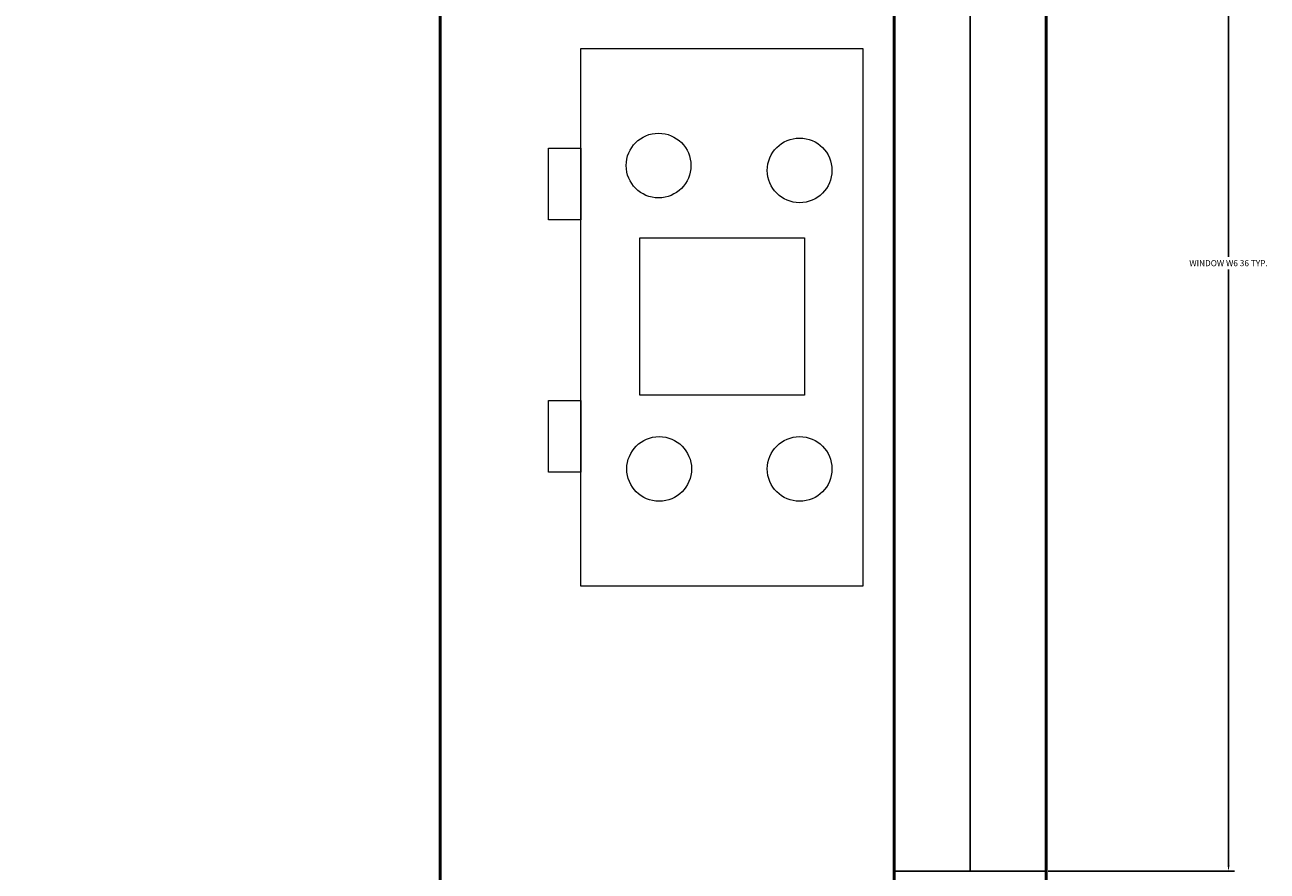
# Model space of a CAD drawing. Units: inches. Extents: x 1901 to 2863, y 888 to 2433.
# Tile 87 of 91: x 2723 to 2759, y 2027 to 2052. Entities that reach past the tile are written whole.
import ezdxf

# ---------------------------------------------------------------- set-up
doc = ezdxf.new("R2010")
doc.units = ezdxf.units.IN
for name, color, linetype, lineweight in [('A-ANNO-DIMS', 2, 'Continuous', 18), ('A-FLOR-FIXT', 9, 'Continuous', 18), ('A-GLAZ', 3, 'Continuous', 25), ('A-WALL', 7, 'Continuous', 50), ('A-WALL-PATT', 8, 'Continuous', 13)]:
    doc.layers.add(name, color=color, linetype=linetype, lineweight=lineweight)
doc.styles.get("Standard").update_dxf_attribs({"font": 'arial.ttf'})
doc.dimstyles.get("Standard").update_dxf_attribs({"dimtxt": 0.18, "dimasz": 0.18, "dimexe": 0.18, "dimexo": 0.0625, "dimgap": 0.09, "dimtad": 0, "dimtih": 1, "dimtoh": 1, "dimdec": 4, "dimzin": 0, "dimdsep": 46, "dimtxsty": 'Standard', "dimcen": 0.09, "dimadec": 0, "dimazin": 0, "dimtfac": 1, "dimtdec": 4, "dimtofl": 0, "dimtmove": 0, "dimatfit": 3, "dimfxl": 1, "dimtolj": 1, "dimtzin": 0, "dimarcsym": 0})

# ---------------------------------------------------------------- blocks, each defined once
blk = doc.blocks.new('WIN-36-5')
for p, q in [((0, 36), (4.5, 36)), ((4.5, 36), (2.25, 36)), ((2.25, 36), (2.25, 0)), ((2.25, 0), (0, 0)), ((0, 0), (4.5, 0))]:
    blk.add_line(p, q)
blk = doc.blocks.new('*D29')
at = {"layer": 'A-ANNO-DIMS', "color": 0, "lineweight": -2, "transparency": 16777216}
for p, q in [((2752.989, 2063.429), (2758.506, 2063.429)), ((2758.326, 2063.249), (2758.326, 2045.612)), ((2758.326, 2027.609), (2758.326, 2045.245)), ((2752.989, 2027.429), (2758.506, 2027.429))]:
    blk.add_line(p, q, dxfattribs=at)
at = {"layer": 'A-ANNO-DIMS', "color": 0, "transparency": 16777216}
for points in [[(2758.296, 2063.249), (2758.356, 2063.249), (2758.326, 2063.429)], [(2758.296, 2027.609), (2758.356, 2027.609), (2758.326, 2027.429)]]:
    blk.add_solid(points, dxfattribs=at)
at = {"layer": 'Defpoints', "color": 0, "transparency": 16777216}
for p in [(2752.926, 2063.429), (2758.326, 2063.429), (2752.926, 2027.429)]:
    blk.add_point(p, dxfattribs=at)
at = {"layer": 'A-ANNO-DIMS', "color": 0, "transparency": 16777216, "insert": (2758.326, 2045.429), "char_height": 0.18, "attachment_point": 5}
blk.add_mtext('\\A1;WINDOW W6 36 TYP.', dxfattribs=at)
blk = doc.blocks.new('*D30')
at = {"layer": 'A-ANNO-DIMS', "color": 0, "lineweight": -2, "transparency": 16777216}
for p, q in [((2748.426, 2027.366), (2748.426, 2021.849)), ((2752.926, 2027.366), (2752.926, 2021.849)), ((2748.606, 2022.029), (2750.218, 2022.029)), ((2752.746, 2022.029), (2751.134, 2022.029))]:
    blk.add_line(p, q, dxfattribs=at)
at = {"layer": 'A-ANNO-DIMS', "color": 0, "transparency": 16777216}
for points in [[(2748.606, 2022.059), (2748.606, 2021.999), (2748.426, 2022.029)], [(2752.746, 2022.059), (2752.746, 2021.999), (2752.926, 2022.029)]]:
    blk.add_solid(points, dxfattribs=at)
at = {"layer": 'Defpoints', "color": 0, "transparency": 16777216}
for p in [(2748.426, 2027.429), (2752.926, 2027.429), (2752.926, 2022.029)]:
    blk.add_point(p, dxfattribs=at)
at = {"layer": 'A-ANNO-DIMS', "color": 0, "transparency": 16777216, "insert": (2750.676, 2022.029), "char_height": 0.18, "attachment_point": 5}
blk.add_mtext('\\A1;5 TYP.', dxfattribs=at)

msp = doc.modelspace()

# ---------------------------------------------------------------- hatches: boundary and pattern name
at = {"layer": 'A-WALL-PATT'}
h = msp.add_hatch(dxfattribs=at)
h.set_pattern_fill('ANSI32', color=256)
h.paths.add_polyline_path([(2192.501, 2274.134), (2141.264, 2274.134), (2141.264, 2269.634), (2192.501, 2269.634)])
h.paths.add_polyline_path([(2259.926, 2274.134), (2216.501, 2274.134), (2216.501, 2269.634), (2255.426, 2269.634), (2255.426, 2214.634), (2250.809, 2214.634), (2250.809, 2210.134), (2259.926, 2210.134), (2259.926, 2215.134), (2271.756, 2215.134), (2271.756, 2217.384), (2271.756, 2219.634), (2259.926, 2219.634)])
h.paths.add_polyline_path([(2171.426, 2269.634), (2166.926, 2269.634), (2166.926, 2219.634), (2121.238, 2219.634), (2121.238, 2215.134), (2166.926, 2215.134), (2166.926, 2083.134), (2161.807, 2083.134), (2161.807, 2078.634), (2171.426, 2078.634), (2176.996, 2078.634), (2176.996, 2080.884), (2176.996, 2083.134), (2171.426, 2083.134), (2171.426, 2210.134), (2230.912, 2210.134), (2230.912, 2212.384), (2230.912, 2214.634), (2171.426, 2214.634)])
h.paths.add_polyline_path([(2117.264, 2274.134), (2089.426, 2274.134), (2089.426, 2219.634), (2081.136, 2219.634), (2081.136, 2215.134), (2089.426, 2215.134), (2098.004, 2215.134), (2098.004, 2217.384), (2098.004, 2219.634), (2093.926, 2219.634), (2093.926, 2269.634), (2117.264, 2269.634), (2117.264, 2271.884)])
h.paths.add_polyline_path([(2343.426, 2219.634), (2329.295, 2219.634), (2329.295, 2215.134), (2338.926, 2215.134), (2338.926, 2184.739), (2343.426, 2184.739)])
h.paths.add_polyline_path([(2338.926, 2083.134), (2329.295, 2083.134), (2208.966, 2083.134), (2208.966, 2078.634), (2338.926, 2078.634)])
h.paths.add_polyline_path([(2343.426, 2136.739), (2338.926, 2136.739), (2338.926, 1872.634), (2343.426, 1872.634)])
h.paths.add_polyline_path([(2343.426, 1863.634), (2397.68, 1863.634), (2397.68, 1821.634), (2384.138, 1821.634), (2384.138, 1812.634), (2418.33, 1812.634), (2418.33, 1817.134), (2418.33, 1821.634), (2406.68, 1821.634), (2406.68, 1863.634), (2459.499, 1863.634), (2459.499, 1821.634), (2447.138, 1821.634), (2447.138, 1812.634), (2459.499, 1812.634), (2468.499, 1812.634), (2468.499, 1872.634), (2394.426, 1872.634), (2334.426, 1872.634), (2334.426, 1812.634), (2343.426, 1812.634), (2353.251, 1812.634), (2353.251, 1821.634), (2343.426, 1821.634)])
h.paths.add_polyline_path([(2510.014, 1872.634), (2468.499, 1872.634), (2468.499, 1868.134), (2510.014, 1868.134)])
h.paths.add_polyline_path([(2514.009, 1817.134), (2468.499, 1817.134), (2468.499, 1812.634), (2482.114, 1812.634), (2482.114, 1800.606), (2486.614, 1800.606), (2486.614, 1812.634), (2514.009, 1812.634)])
h.paths.add_polyline_path([(2299.247, 1814.884), (2299.247, 1817.134), (2295.926, 1817.134), (2295.926, 1854.169), (2293.676, 1854.169), (2291.426, 1854.169), (2291.426, 1817.134), (2266.109, 1817.134), (2266.109, 1812.634), (2299.247, 1812.634)])
h.paths.add_polyline_path([(2218.109, 1817.134), (2206.46, 1817.134), (2171.426, 1817.134), (2171.426, 1949.134), (2190.1, 1949.134), (2190.1, 1953.634), (2163.468, 1953.634), (2163.468, 1949.134), (2166.926, 1949.134), (2166.926, 1817.134), (2114.297, 1817.134), (2114.297, 1812.634), (2218.109, 1812.634)])
h.paths.add_polyline_path([(2029.426, 1970.922), (2024.926, 1970.922), (2024.926, 1912.717), (2029.426, 1912.717)])
h.paths.add_polyline_path([(2132.297, 1953.634), (2113.926, 1953.634), (2113.926, 1975.888), (2111.676, 1975.888), (2109.426, 1975.888), (2109.426, 1953.634), (2029.426, 1953.634), (2029.426, 1949.134), (2132.297, 1949.134)])
h.paths.add_polyline_path([(2029.426, 1853.606), (2029.31, 1853.606), (2029.31, 1853.606), (2029.426, 1853.606), (2029.426, 1864.717), (2024.926, 1864.717), (2024.926, 1812.634), (2066.297, 1812.634), (2066.297, 1814.884), (2066.297, 1817.134), (2029.426, 1817.134)])
h.paths.add_polyline_path([(2122.926, 2010.088), (2120.676, 2010.088), (2118.426, 2010.088), (2118.426, 2006.134), (2029.426, 2006.134), (2029.426, 2001.634), (2109.426, 2001.634), (2109.426, 1998.041), (2113.926, 1998.041), (2113.926, 2001.634), (2122.926, 2001.634)])
h.paths.add_polyline_path([(2029.426, 2031.376), (2024.926, 2031.376), (2024.926, 1994.922), (2027.176, 1994.922), (2029.426, 1994.922)])
h.paths.add_polyline_path([(2029.426, 2136.739), (2024.926, 2136.739), (2024.926, 2067.376), (2027.176, 2067.376), (2029.426, 2067.376)])
h.paths.add_polyline_path([(2125.618, 2083.134), (2029.426, 2083.134), (2029.426, 2078.634), (2118.426, 2078.634), (2118.426, 2030.715), (2122.926, 2030.715), (2122.926, 2078.634), (2125.618, 2078.634)])
h.paths.add_polyline_path([(2029.426, 2215.134), (2040.468, 2215.134), (2040.468, 2217.384), (2040.468, 2219.634), (2024.926, 2219.634), (2024.926, 2184.739), (2029.426, 2184.739), (2029.426, 2187.778)])
h.paths.add_polyline_path([(2686.426, 2274.134), (2659.284, 2274.134), (2659.284, 2269.634), (2681.926, 2269.634), (2681.926, 2219.634), (2676.816, 2219.634), (2676.816, 2215.134), (2681.926, 2215.134), (2697.011, 2215.134), (2697.011, 2217.384), (2697.011, 2219.634), (2686.426, 2219.634)])
h.paths.add_polyline_path([(2609.926, 2269.634), (2635.284, 2269.634), (2635.284, 2274.134), (2571.431, 2274.134), (2571.431, 2269.634), (2605.426, 2269.634), (2605.426, 2214.634), (2549.098, 2214.634), (2549.098, 2210.134), (2605.426, 2210.134), (2605.426, 2083.134), (2601.014, 2083.134), (2601.014, 2080.884), (2601.014, 2078.634), (2609.926, 2078.634), (2616.162, 2078.634), (2616.162, 2080.884), (2616.162, 2083.134), (2609.926, 2083.134), (2609.926, 2215.134), (2651.465, 2215.134), (2651.465, 2217.384), (2651.465, 2219.634), (2609.926, 2219.634)])
h.paths.add_polyline_path([(2521.426, 2269.634), (2547.431, 2269.634), (2547.431, 2271.884), (2547.431, 2274.134), (2516.926, 2274.134), (2516.926, 2219.634), (2506.41, 2219.634), (2506.41, 2215.134), (2516.926, 2215.134), (2516.926, 2210.134), (2525.402, 2210.134), (2525.402, 2212.384), (2525.402, 2214.634), (2521.426, 2214.634)])
h.paths.add_polyline_path([(2456.011, 2219.634), (2439.426, 2219.634), (2439.426, 2187.888), (2443.926, 2187.888), (2443.926, 2215.134), (2456.011, 2215.134)])
h.paths.add_polyline_path([(2752.926, 2219.634), (2739.485, 2219.634), (2739.485, 2215.134), (2748.426, 2215.134), (2748.426, 2187.888), (2752.926, 2187.888)])
h.paths.add_polyline_path([(2752.926, 2139.888), (2748.426, 2139.888), (2748.426, 2083.134), (2648.416, 2083.134), (2648.416, 2078.634), (2654.926, 2078.634), (2654.926, 2039.437), (2659.426, 2039.437), (2659.426, 2078.634), (2748.426, 2078.634), (2748.426, 2063.429), (2752.926, 2063.429)])
h.paths.add_polyline_path([(2752.926, 2010.634), (2659.426, 2010.634), (2659.426, 2015.652), (2654.926, 2015.652), (2654.926, 2010.634), (2605.426, 2010.634), (2605.426, 1920.967), (2609.926, 1920.967), (2609.926, 2006.134), (2748.426, 2006.134), (2748.426, 1982.466), (2752.926, 1982.466)])
h.paths.add_polyline_path([(2752.926, 2027.429), (2748.426, 2027.429), (2748.426, 2010.634), (2752.926, 2010.634)])
h.paths.add_polyline_path([(2748.426, 1886.134), (2609.926, 1886.134), (2609.926, 1889.719), (2605.426, 1889.719), (2605.426, 1861.262), (2609.926, 1861.262), (2609.926, 1881.634), (2748.426, 1881.634)])
h.paths.add_polyline_path([(2456.855, 2228.831), (2498.401, 2228.831), (2498.401, 2247.488), (2456.855, 2247.488)], flags=9)
h.paths.add_polyline_path([(2038.602, 2237.418), (2080.174, 2237.418), (2080.174, 2256.075), (2038.602, 2256.075)], flags=9)
h.paths.add_polyline_path([(2292.009, 1062.394), (2539.932, 1062.394), (2539.932, 1099.487), (2292.009, 1099.487)], flags=9)
h.paths.add_polyline_path([(2424.91, 1832.253), (2448.513, 1832.253), (2448.513, 1846.678), (2424.91, 1846.678)], flags=25)
h.paths.add_polyline_path([(2359.076, 1832.253), (2382.678, 1832.253), (2382.678, 1846.678), (2359.076, 1846.678)], flags=25)
h.paths.add_polyline_path([(2352.899, 1684.802), (2367.543, 1684.802), (2367.543, 1697.167), (2352.899, 1697.167)], flags=9)
h.paths.add_polyline_path([(2079.288, 1755.826), (2169.024, 1755.826), (2169.024, 1774.372), (2079.288, 1774.372)], flags=9)
h.paths.add_polyline_path([(2404.09, 1373.857), (2404.09, 1463.593), (2385.544, 1463.593), (2385.544, 1373.857)], flags=9)
h.paths.add_polyline_path([(2268.091, 2236.371), (2309.636, 2236.371), (2309.636, 2255.028), (2268.091, 2255.028)], flags=9)
h.paths.add_polyline_path([(2575.96, 1700.951), (2665.696, 1700.951), (2665.696, 1719.498), (2575.96, 1719.498)], flags=9)
h.paths.add_polyline_path([(2302.962, 1878.474), (2329.524, 1878.474), (2329.524, 1888.777), (2302.962, 1888.777)], flags=9)
h.paths.add_polyline_path([(2097.415, 2240.576), (2126.573, 2240.576), (2126.573, 2259.233), (2097.415, 2259.233)], flags=9)
h.paths.add_polyline_path([(2208.725, 2246.124), (2237.882, 2246.124), (2237.882, 2264.781), (2208.725, 2264.781)], flags=9)
h.paths.add_polyline_path([(2038.147, 1925.958), (2076.987, 1925.958), (2076.987, 1944.615), (2038.147, 1944.615)], flags=9)
h.paths.add_polyline_path([(2239.144, 1926.672), (2288.465, 1926.672), (2288.465, 1945.329), (2239.144, 1945.329)], flags=9)
h.paths.add_polyline_path([(2175.429, 2007.33), (2212.356, 2007.33), (2212.356, 2025.987), (2175.429, 2025.987)], flags=9)
h.paths.add_polyline_path([(2225.034, 2091.794), (2263.875, 2091.794), (2263.875, 2110.451), (2225.034, 2110.451)], flags=9)
h.paths.add_polyline_path([(2035.398, 2098.478), (2074.238, 2098.478), (2074.238, 2117.135), (2035.398, 2117.135)], flags=9)
h.paths.add_polyline_path([(2050.102, 2029.209), (2083.26, 2029.209), (2083.26, 2047.866), (2050.102, 2047.866)], flags=9)
h.paths.add_polyline_path([(2069.677, 1956.719), (2098.835, 1956.719), (2098.835, 1975.376), (2069.677, 1975.376)], flags=25)
h.paths.add_polyline_path([(2328.62, 1753.336), (2361.663, 1753.336), (2361.663, 1771.993), (2328.62, 1771.993)], flags=9)
h.paths.add_polyline_path([(2395.162, 2060.888), (2395.162, 2140.654), (2378.676, 2140.654), (2378.676, 2060.888)], flags=9)
h.paths.add_polyline_path([(2463.728, 2059.02), (2492.886, 2059.02), (2492.886, 2077.677), (2463.728, 2077.677)], flags=9)
h.paths.add_polyline_path([(2458.027, 2181.536), (2496.868, 2181.536), (2496.868, 2200.194), (2458.027, 2200.194)], flags=9)
h.paths.add_polyline_path([(2527.577, 2243.074), (2556.735, 2243.074), (2556.735, 2261.731), (2527.577, 2261.731)], flags=9)
h.paths.add_polyline_path([(2694.461, 2232.767), (2736.033, 2232.767), (2736.033, 2251.425), (2694.461, 2251.425)], flags=9)
h.paths.add_polyline_path([(2637.821, 2249.225), (2666.979, 2249.225), (2666.979, 2267.882), (2637.821, 2267.882)], flags=9)
h.paths.add_polyline_path([(2623.687, 2183.541), (2662.528, 2183.541), (2662.528, 2202.199), (2623.687, 2202.199)], flags=9)
h.paths.add_polyline_path([(2691.965, 2021.5), (2725.124, 2021.5), (2725.124, 2040.157), (2691.965, 2040.157)], flags=9)
h.paths.add_polyline_path([(2621.043, 1975.912), (2662.335, 1975.912), (2662.335, 1994.569), (2621.043, 1994.569)], flags=25)
h.paths.add_polyline_path([(2479.032, 1927.62), (2519.844, 1927.62), (2519.844, 1946.277), (2479.032, 1946.277)], flags=9)
h.paths.add_polyline_path([(2670.941, 1849.076), (2716.005, 1849.076), (2716.005, 1867.734), (2670.941, 1867.734)], flags=9)
h.paths.add_polyline_path([(2523.613, 1782.956), (2550.175, 1782.956), (2550.175, 1793.26), (2523.613, 1793.26)], flags=9)
h.paths.add_polyline_path([(2450.841, 1207.331), (2492.386, 1207.331), (2492.386, 1225.989), (2450.841, 1225.989)], flags=9)
h.paths.add_polyline_path([(2527.751, 1203.841), (2556.908, 1203.841), (2556.908, 1222.499), (2527.751, 1222.499)], flags=9)
h.paths.add_polyline_path([(2639.111, 1207.2), (2668.268, 1207.2), (2668.268, 1225.857), (2639.111, 1225.857)], flags=9)
h.paths.add_polyline_path([(2692.594, 1218.965), (2734.167, 1218.965), (2734.167, 1237.623), (2692.594, 1237.623)], flags=9)
h.paths.add_polyline_path([(2669.266, 1366.329), (2708.106, 1366.329), (2708.106, 1384.987), (2669.266, 1384.987)], flags=9)
h.paths.add_polyline_path([(2463.313, 1358.031), (2502.153, 1358.031), (2502.153, 1376.688), (2463.313, 1376.688)], flags=9)
h.paths.add_polyline_path([(2494.725, 1449.963), (2531.652, 1449.963), (2531.652, 1468.62), (2494.725, 1468.62)], flags=9)
h.paths.add_polyline_path([(2675.565, 1422.157), (2708.724, 1422.157), (2708.724, 1440.815), (2675.565, 1440.815)], flags=9)
h.paths.add_polyline_path([(2685.634, 1493.891), (2714.792, 1493.891), (2714.792, 1512.548), (2685.634, 1512.548)], flags=9)
h.paths.add_polyline_path([(2686.805, 1529.913), (2725.645, 1529.913), (2725.645, 1548.57), (2686.805, 1548.57)], flags=9)
h.paths.add_polyline_path([(2503.651, 1537.991), (2552.972, 1537.991), (2552.972, 1556.648), (2503.651, 1556.648)], flags=9)
h.paths.add_polyline_path([(2291.713, 1643.504), (2318.275, 1643.504), (2318.275, 1653.807), (2291.713, 1653.807)], flags=9)
h.paths.add_polyline_path([(2450.626, 1610.52), (2477.189, 1610.52), (2477.189, 1620.824), (2450.626, 1620.824)], flags=9)
h.paths.add_polyline_path([(2359.985, 1551.814), (2422.253, 1551.814), (2422.253, 1562.117), (2359.985, 1562.117)], flags=9)
h.paths.add_polyline_path([(2280.106, 1249.006), (2321.651, 1249.006), (2321.651, 1267.663), (2280.106, 1267.663)], flags=9)
h.paths.add_polyline_path([(2164.057, 1274.232), (2193.215, 1274.232), (2193.215, 1292.889), (2164.057, 1292.889)], flags=9)
h.paths.add_polyline_path([(2118.21, 1277.694), (2151.252, 1277.694), (2151.252, 1296.351), (2118.21, 1296.351)], flags=9)
h.paths.add_polyline_path([(2031.946, 1268.529), (2073.519, 1268.529), (2073.519, 1287.187), (2031.946, 1287.187)], flags=9)
h.paths.add_polyline_path([(2050.199, 1409.079), (2089.04, 1409.079), (2089.04, 1427.736), (2050.199, 1427.736)], flags=9)
h.paths.add_polyline_path([(2243.743, 1421.032), (2282.584, 1421.032), (2282.584, 1439.689), (2243.743, 1439.689)], flags=9)
h.paths.add_polyline_path([(2190.746, 1509.769), (2231.558, 1509.769), (2231.558, 1528.426), (2190.746, 1528.426)], flags=9)
h.paths.add_polyline_path([(2058.392, 1475.415), (2091.55, 1475.415), (2091.55, 1494.073), (2058.392, 1494.073)], flags=9)
h.paths.add_polyline_path([(2062.447, 1553.09), (2091.605, 1553.09), (2091.605, 1571.747), (2062.447, 1571.747)], flags=9)
h.paths.add_polyline_path([(2219.524, 1590.365), (2266.147, 1590.365), (2266.147, 1609.022), (2219.524, 1609.022)], flags=9)
h.paths.add_polyline_path([(2041.072, 1584.188), (2079.912, 1584.188), (2079.912, 1602.845), (2041.072, 1602.845)], flags=9)
h = msp.add_hatch(dxfattribs=at)
h.set_pattern_fill('ANSI32', color=256)
h.paths.add_polyline_path([(2443.926, 2139.888), (2439.426, 2139.888), (2439.426, 2069.348), (2441.676, 2069.348), (2443.926, 2069.348), (2443.926, 2078.634), (2521.926, 2078.634), (2521.926, 2075.067), (2524.176, 2075.067), (2526.426, 2075.067), (2526.426, 2078.634), (2571.755, 2078.634), (2571.755, 2080.884), (2571.755, 2083.134), (2443.926, 2083.134)])
h.paths.add_polyline_path([(2526.426, 2054.634), (2524.176, 2054.634), (2521.926, 2054.634), (2521.926, 2030.634), (2443.926, 2030.634), (2443.926, 2045.348), (2439.426, 2045.348), (2439.426, 1983.867), (2443.926, 1983.867), (2443.926, 2026.134), (2521.926, 2026.134), (2526.426, 2026.134)])
h.paths.add_polyline_path([(2443.926, 1923.867), (2439.426, 1923.867), (2439.426, 1872.634), (2443.926, 1872.634)])
h.paths.add_polyline_path([(2636.233, 1766.134), (2609.926, 1766.134), (2609.926, 1779.785), (2605.426, 1779.785), (2605.426, 1766.134), (2486.614, 1766.134), (2486.614, 1770.671), (2482.114, 1770.671), (2482.114, 1766.134), (2482.114, 1761.634), (2636.233, 1761.634), (2636.233, 1763.884)])
h.paths.add_polyline_path([(2519.536, 1663.384), (2519.536, 1665.634), (2494.926, 1665.634), (2481.831, 1665.634), (2481.831, 1663.384), (2481.831, 1661.134), (2490.426, 1661.134), (2490.426, 1640.157), (2494.926, 1640.157), (2494.926, 1661.134), (2519.536, 1661.134)])
h.paths.add_polyline_path([(2443.926, 1712.134), (2443.926, 1716.634), (2414.464, 1716.634), (2414.464, 1712.134), (2439.426, 1712.134), (2439.426, 1545.507), (2443.926, 1545.507), (2443.926, 1661.134), (2448.475, 1661.134), (2448.475, 1665.634), (2443.926, 1665.634)])
h.paths.add_polyline_path([(2343.426, 1712.134), (2365.525, 1712.134), (2365.525, 1714.384), (2365.525, 1716.634), (2333.871, 1716.634), (2333.871, 1714.384), (2333.871, 1712.134), (2338.926, 1712.134), (2338.926, 1575.634), (2338.926, 1545.507), (2343.426, 1545.507), (2343.426, 1547.507), (2343.426, 1580.134)])
h.paths.add_polyline_path([(2752.926, 1665.634), (2579.536, 1665.634), (2579.536, 1661.134), (2615.926, 1661.134), (2615.926, 1529.134), (2598.931, 1529.134), (2598.931, 1524.634), (2623.127, 1524.634), (2623.127, 1526.884), (2623.127, 1529.134), (2620.426, 1529.134), (2620.426, 1661.134), (2748.426, 1661.134), (2748.426, 1633.499), (2752.926, 1633.499)])
h.paths.add_polyline_path([(2752.926, 1419.929), (2748.426, 1419.929), (2748.426, 1400.134), (2659.426, 1400.134), (2659.426, 1444.333), (2657.176, 1444.333), (2654.926, 1444.333), (2654.926, 1400.134), (2643.649, 1400.134), (2643.649, 1395.634), (2748.426, 1395.634), (2748.426, 1364.035), (2752.926, 1364.035)])
h.paths.add_polyline_path([(2752.926, 1492.878), (2748.426, 1492.878), (2748.426, 1476.634), (2667.426, 1476.634), (2667.426, 1479.71), (2665.176, 1479.71), (2662.926, 1479.71), (2662.926, 1476.634), (2654.926, 1476.634), (2654.926, 1469.536), (2659.426, 1469.536), (2659.426, 1472.134), (2748.426, 1472.134), (2748.426, 1455.929), (2752.926, 1455.929)])
h.paths.add_polyline_path([(2752.926, 1304.035), (2748.426, 1304.035), (2748.426, 1263.634), (2738.66, 1263.634), (2738.66, 1259.134), (2752.926, 1259.134)])
h.paths.add_polyline_path([(2685.926, 1259.134), (2695.49, 1259.134), (2695.49, 1261.384), (2695.49, 1263.634), (2677.837, 1263.634), (2677.837, 1261.384), (2677.837, 1259.134), (2681.426, 1259.134), (2681.426, 1203.634), (2653.277, 1203.634), (2653.277, 1199.134), (2685.926, 1199.134), (2685.926, 1203.634)])
h.paths.add_polyline_path([(2609.426, 1395.634), (2611.848, 1395.634), (2611.848, 1400.134), (2598.888, 1400.134), (2598.888, 1397.884), (2598.888, 1395.634), (2604.926, 1395.634), (2604.926, 1268.134), (2554.726, 1268.134), (2554.726, 1265.884), (2554.726, 1263.634), (2604.926, 1263.634), (2604.926, 1203.634), (2571.306, 1203.634), (2571.306, 1199.134), (2604.926, 1199.134), (2629.277, 1199.134), (2629.277, 1201.384), (2629.277, 1203.634), (2609.426, 1203.634), (2609.426, 1258.634), (2609.426, 1259.134), (2654.804, 1259.134), (2654.804, 1263.634), (2609.426, 1263.634)])
h.paths.add_polyline_path([(2443.926, 1304.035), (2439.426, 1304.035), (2439.426, 1259.134), (2443.926, 1259.134), (2456.16, 1259.134), (2456.16, 1261.384), (2456.16, 1263.634), (2443.926, 1263.634)])
h.paths.add_polyline_path([(2525.426, 1263.634), (2531.778, 1263.634), (2531.778, 1268.134), (2520.926, 1268.134), (2520.926, 1263.634), (2511.409, 1263.634), (2511.409, 1259.134), (2520.926, 1259.134), (2520.926, 1199.134), (2547.306, 1199.134), (2547.306, 1201.384), (2547.306, 1203.634), (2525.426, 1203.634)])
h.paths.add_polyline_path([(2443.926, 1434.842), (2439.426, 1434.842), (2439.426, 1364.035), (2441.676, 1364.035), (2443.926, 1364.035)])
h.paths.add_polyline_path([(2567.134, 1400.134), (2443.926, 1400.134), (2443.926, 1395.634), (2567.134, 1395.634)])
h.paths.add_polyline_path([(2443.926, 1545.507), (2439.426, 1545.507), (2439.426, 1494.842), (2443.926, 1494.842)])
h.paths.add_polyline_path([(2494.926, 1553.349), (2492.676, 1553.349), (2490.426, 1553.349), (2490.426, 1524.634), (2494.926, 1524.634), (2525.936, 1524.634), (2525.936, 1526.884), (2525.936, 1529.134), (2494.926, 1529.134)])
h.paths.add_polyline_path([(2752.926, 1573.499), (2748.426, 1573.499), (2748.426, 1529.134), (2657.759, 1529.134), (2657.759, 1524.634), (2662.926, 1524.634), (2662.926, 1498.631), (2667.426, 1498.631), (2667.426, 1524.634), (2748.426, 1524.634), (2748.426, 1516.878), (2752.926, 1516.878)])
h.paths.add_polyline_path([(2038.602, 2237.418), (2080.174, 2237.418), (2080.174, 2256.075), (2038.602, 2256.075)], flags=9)
h.paths.add_polyline_path([(2292.009, 1062.394), (2539.932, 1062.394), (2539.932, 1099.487), (2292.009, 1099.487)], flags=9)
h.paths.add_polyline_path([(2424.91, 1832.253), (2448.513, 1832.253), (2448.513, 1846.678), (2424.91, 1846.678)], flags=9)
h.paths.add_polyline_path([(2359.076, 1832.253), (2382.678, 1832.253), (2382.678, 1846.678), (2359.076, 1846.678)], flags=9)
h.paths.add_polyline_path([(2352.899, 1684.802), (2367.543, 1684.802), (2367.543, 1697.167), (2352.899, 1697.167)], flags=9)
h.paths.add_polyline_path([(2079.288, 1755.826), (2169.024, 1755.826), (2169.024, 1774.372), (2079.288, 1774.372)], flags=9)
h.paths.add_polyline_path([(2404.09, 1373.857), (2404.09, 1463.593), (2385.544, 1463.593), (2385.544, 1373.857)], flags=9)
h.paths.add_polyline_path([(2268.091, 2236.371), (2309.636, 2236.371), (2309.636, 2255.028), (2268.091, 2255.028)], flags=9)
h.paths.add_polyline_path([(2575.96, 1700.951), (2665.696, 1700.951), (2665.696, 1719.498), (2575.96, 1719.498)], flags=9)
h.paths.add_polyline_path([(2302.962, 1878.474), (2329.524, 1878.474), (2329.524, 1888.777), (2302.962, 1888.777)], flags=9)
h.paths.add_polyline_path([(2097.415, 2240.576), (2126.573, 2240.576), (2126.573, 2259.233), (2097.415, 2259.233)], flags=9)
h.paths.add_polyline_path([(2208.725, 2246.124), (2237.882, 2246.124), (2237.882, 2264.781), (2208.725, 2264.781)], flags=9)
h.paths.add_polyline_path([(2038.147, 1925.958), (2076.987, 1925.958), (2076.987, 1944.615), (2038.147, 1944.615)], flags=9)
h.paths.add_polyline_path([(2239.144, 1926.672), (2288.465, 1926.672), (2288.465, 1945.329), (2239.144, 1945.329)], flags=9)
h.paths.add_polyline_path([(2175.429, 2007.33), (2212.356, 2007.33), (2212.356, 2025.987), (2175.429, 2025.987)], flags=9)
h.paths.add_polyline_path([(2225.034, 2091.794), (2263.875, 2091.794), (2263.875, 2110.451), (2225.034, 2110.451)], flags=9)
h.paths.add_polyline_path([(2035.398, 2098.478), (2074.238, 2098.478), (2074.238, 2117.135), (2035.398, 2117.135)], flags=9)
h.paths.add_polyline_path([(2050.102, 2029.209), (2083.26, 2029.209), (2083.26, 2047.866), (2050.102, 2047.866)], flags=9)
h.paths.add_polyline_path([(2069.677, 1956.719), (2098.835, 1956.719), (2098.835, 1975.376), (2069.677, 1975.376)], flags=9)
h.paths.add_polyline_path([(2328.62, 1753.336), (2361.663, 1753.336), (2361.663, 1771.993), (2328.62, 1771.993)], flags=9)
h.paths.add_polyline_path([(2395.162, 2060.888), (2395.162, 2140.654), (2378.676, 2140.654), (2378.676, 2060.888)], flags=9)
h.paths.add_polyline_path([(2463.728, 2059.02), (2492.886, 2059.02), (2492.886, 2077.677), (2463.728, 2077.677)], flags=9)
h.paths.add_polyline_path([(2458.027, 2181.536), (2496.868, 2181.536), (2496.868, 2200.194), (2458.027, 2200.194)], flags=9)
h.paths.add_polyline_path([(2456.855, 2228.831), (2498.401, 2228.831), (2498.401, 2247.488), (2456.855, 2247.488)], flags=9)
h.paths.add_polyline_path([(2527.577, 2243.074), (2556.735, 2243.074), (2556.735, 2261.731), (2527.577, 2261.731)], flags=9)
h.paths.add_polyline_path([(2694.461, 2232.767), (2736.033, 2232.767), (2736.033, 2251.425), (2694.461, 2251.425)], flags=9)
h.paths.add_polyline_path([(2637.821, 2249.225), (2666.979, 2249.225), (2666.979, 2267.882), (2637.821, 2267.882)], flags=9)
h.paths.add_polyline_path([(2623.687, 2183.541), (2662.528, 2183.541), (2662.528, 2202.199), (2623.687, 2202.199)], flags=9)
h.paths.add_polyline_path([(2691.965, 2021.5), (2725.124, 2021.5), (2725.124, 2040.157), (2691.965, 2040.157)], flags=9)
h.paths.add_polyline_path([(2621.043, 1975.912), (2662.335, 1975.912), (2662.335, 1994.569), (2621.043, 1994.569)], flags=9)
h.paths.add_polyline_path([(2479.032, 1927.62), (2519.844, 1927.62), (2519.844, 1946.277), (2479.032, 1946.277)], flags=9)
h.paths.add_polyline_path([(2670.941, 1849.076), (2716.005, 1849.076), (2716.005, 1867.734), (2670.941, 1867.734)], flags=9)
h.paths.add_polyline_path([(2523.613, 1782.956), (2550.175, 1782.956), (2550.175, 1793.26), (2523.613, 1793.26)], flags=9)
h.paths.add_polyline_path([(2450.841, 1207.331), (2492.386, 1207.331), (2492.386, 1225.989), (2450.841, 1225.989)], flags=9)
h.paths.add_polyline_path([(2527.751, 1203.841), (2556.908, 1203.841), (2556.908, 1222.499), (2527.751, 1222.499)], flags=9)
h.paths.add_polyline_path([(2639.111, 1207.2), (2668.268, 1207.2), (2668.268, 1225.857), (2639.111, 1225.857)], flags=9)
h.paths.add_polyline_path([(2692.594, 1218.965), (2734.167, 1218.965), (2734.167, 1237.623), (2692.594, 1237.623)], flags=9)
h.paths.add_polyline_path([(2669.266, 1366.329), (2708.106, 1366.329), (2708.106, 1384.987), (2669.266, 1384.987)], flags=25)
h.paths.add_polyline_path([(2463.313, 1358.031), (2502.153, 1358.031), (2502.153, 1376.688), (2463.313, 1376.688)], flags=9)
h.paths.add_polyline_path([(2494.725, 1449.963), (2531.652, 1449.963), (2531.652, 1468.62), (2494.725, 1468.62)], flags=9)
h.paths.add_polyline_path([(2675.565, 1422.157), (2708.724, 1422.157), (2708.724, 1440.815), (2675.565, 1440.815)], flags=25)
h.paths.add_polyline_path([(2685.634, 1493.891), (2714.792, 1493.891), (2714.792, 1512.548), (2685.634, 1512.548)], flags=9)
h.paths.add_polyline_path([(2686.805, 1529.913), (2725.645, 1529.913), (2725.645, 1548.57), (2686.805, 1548.57)], flags=25)
h.paths.add_polyline_path([(2503.651, 1537.991), (2552.972, 1537.991), (2552.972, 1556.648), (2503.651, 1556.648)], flags=9)
h.paths.add_polyline_path([(2291.713, 1643.504), (2318.275, 1643.504), (2318.275, 1653.807), (2291.713, 1653.807)], flags=9)
h.paths.add_polyline_path([(2450.626, 1610.52), (2477.189, 1610.52), (2477.189, 1620.824), (2450.626, 1620.824)], flags=9)
h.paths.add_polyline_path([(2359.985, 1551.814), (2422.253, 1551.814), (2422.253, 1562.117), (2359.985, 1562.117)], flags=9)
h.paths.add_polyline_path([(2280.106, 1249.006), (2321.651, 1249.006), (2321.651, 1267.663), (2280.106, 1267.663)], flags=9)
h.paths.add_polyline_path([(2164.057, 1274.232), (2193.215, 1274.232), (2193.215, 1292.889), (2164.057, 1292.889)], flags=9)
h.paths.add_polyline_path([(2118.21, 1277.694), (2151.252, 1277.694), (2151.252, 1296.351), (2118.21, 1296.351)], flags=9)
h.paths.add_polyline_path([(2031.946, 1268.529), (2073.519, 1268.529), (2073.519, 1287.187), (2031.946, 1287.187)], flags=9)
h.paths.add_polyline_path([(2050.199, 1409.079), (2089.04, 1409.079), (2089.04, 1427.736), (2050.199, 1427.736)], flags=9)
h.paths.add_polyline_path([(2243.743, 1421.032), (2282.584, 1421.032), (2282.584, 1439.689), (2243.743, 1439.689)], flags=9)
h.paths.add_polyline_path([(2190.746, 1509.769), (2231.558, 1509.769), (2231.558, 1528.426), (2190.746, 1528.426)], flags=9)
h.paths.add_polyline_path([(2058.392, 1475.415), (2091.55, 1475.415), (2091.55, 1494.073), (2058.392, 1494.073)], flags=9)
h.paths.add_polyline_path([(2062.447, 1553.09), (2091.605, 1553.09), (2091.605, 1571.747), (2062.447, 1571.747)], flags=9)
h.paths.add_polyline_path([(2219.524, 1590.365), (2266.147, 1590.365), (2266.147, 1609.022), (2219.524, 1609.022)], flags=9)
h.paths.add_polyline_path([(2041.072, 1584.188), (2079.912, 1584.188), (2079.912, 1602.845), (2041.072, 1602.845)], flags=9)

# ---------------------------------------------------------------- linework, layer by layer
at = {"layer": 'A-FLOR-FIXT'}
for points in [[(2747.496, 2035.862), (2739.144, 2035.862), (2739.144, 2051.782), (2747.496, 2051.782)], [(2739.144, 2046.712), (2738.195, 2046.712), (2738.195, 2048.831), (2739.144, 2048.831)], [(2745.774, 2041.522), (2740.899, 2041.522), (2740.899, 2046.18), (2745.774, 2046.18)], [(2739.144, 2039.243), (2738.195, 2039.243), (2738.195, 2041.362), (2739.144, 2041.362)]]:
    msp.add_lwpolyline(points, close=True, dxfattribs=at)
for centre in [(2741.449, 2048.32), (2745.626, 2048.176), (2741.467, 2039.337), (2745.626, 2039.337)]:
    msp.add_circle(centre, 0.958, dxfattribs=at)
at = {"layer": 'A-WALL'}
for p, q in [((2752.926, 2219.634), (2752.926, 1812.634)), ((2748.426, 2078.634), (2748.426, 2010.634)), ((2734.984, 2065.199), (2734.984, 2010.634))]:
    msp.add_line(p, q, dxfattribs=at)

# ---------------------------------------------------------------- block references
at = {"layer": 'A-GLAZ'}
msp.add_blockref('WIN-36-5', (2748.426, 2027.429), dxfattribs=at)

# ---------------------------------------------------------------- dimensions: what is measured, and where the dimension line sits
at = {"layer": 'A-ANNO-DIMS'}
dim = msp.add_linear_dim(base=(2758.326, 2063.429), p1=(2752.926, 2027.429), p2=(2752.926, 2063.429), angle=90, text='WINDOW W6 <> TYP.', dimstyle='Standard', override={"dimdec": 0, "dimlfac": 1, "dimrnd": 0, "dimzin": 0, "dimdsep": 46, "dimlunit": 2}, dxfattribs=at)
dim.commit()
dim.dimension.update_dxf_attribs({"geometry": '*D29', "text_midpoint": (2758.326, 2045.429)})
dim = msp.add_linear_dim(base=(2752.926174575, 2022.028519883), p1=(2748.426174575, 2027.428519883), p2=(2752.926174575, 2027.428519883), text='<> TYP.', dimstyle='Standard', override={"dimdec": 0, "dimlfac": 1, "dimrnd": 0, "dimzin": 0, "dimdsep": 46, "dimlunit": 2}, dxfattribs=at)
dim.commit()
dim.dimension.update_dxf_attribs({"geometry": '*D30', "text_midpoint": (2750.676174575, 2022.028519883)})

doc.saveas('drawing.dxf')
